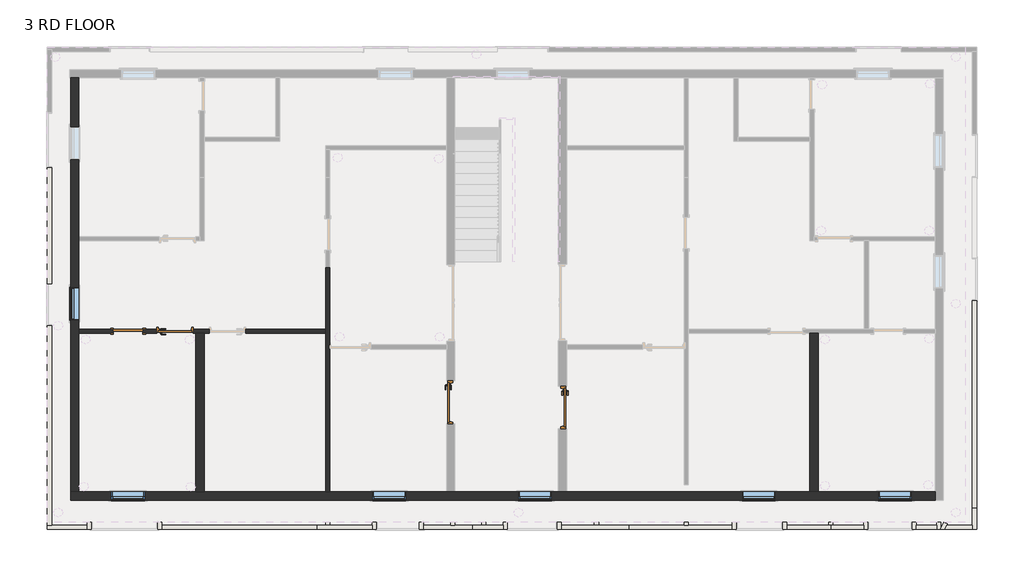
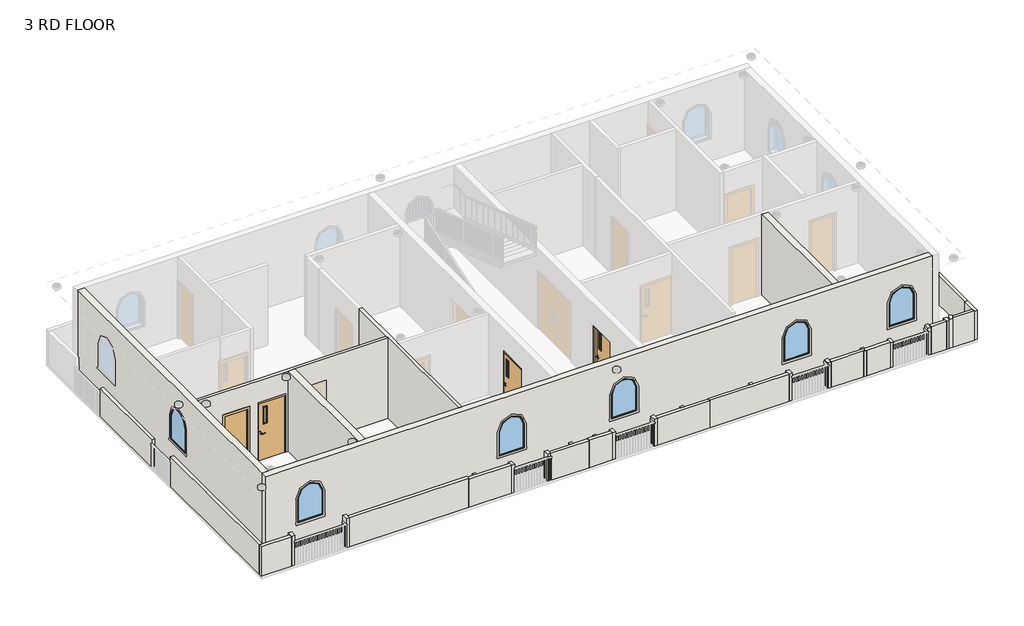
# One storey, part 1 of 7: 39 walls, 6 windows, 4 doors.
"""IFC4 building model written with IfcOpenShell, lengths in millimetres."""

from ifc_helpers import new_model, si_unit, frame, origin, place, context, project, spatial, polyline, circle_curve, outline, extrude, faceted_brep, transform, mapped, element, save
from ifc_brep_helpers import plane_surface, revolved_surface, advanced_brep
from components import door_586e558e, door_7d8f8091, door_passage_single_vision_lite_3_x7_38248cdf, door_d141acb4, window_fixed_round_top_3_x_4_dee2be1c

model = new_model("IFC4")

# Units and contexts
model_context = context("Model", 3, world=origin())
ifc_project = project(units=[si_unit("LENGTHUNIT", "METRE", prefix="MILLI")], contexts=[model_context])

# Site, building, storey
site = spatial("IfcSite", under=ifc_project)
building = spatial("IfcBuilding", under=site)
storey = spatial("IfcBuildingStorey", under=building, Name="3 RD FLOOR", Elevation=9601.2)

# Doors
placement = place(None, origin())
door_shape = door_586e558e(model_context)
element("IfcDoor", 1, ObjectType="Door-Passage-Single-Vision_Lite : 3'6\"X7' 2", at=placement, inside=storey, context=model_context, shape_type="MappedRepresentation", body=[
    mapped(door_shape, transform((1116.1432011, -1461.3932193, 9601.2), x_axis=(0.0, -1.0, 0.0), y_axis=(1.0, 0.0, 0.0), z_axis=(0.0, 0.0, 1.0))),
])
door_2_shape = door_7d8f8091(model_context)
element("IfcDoor", 2, ObjectType="Door-Passage-Single-Vision_Lite : 3'7\"X7' 3", at=placement, inside=storey, context=model_context, shape_type="MappedRepresentation", body=[
    mapped(door_2_shape, transform((-1956.7487998, -1318.7421379, 9601.2), x_axis=(0.0, -1.0, 0.0), y_axis=(1.0, 0.0, 0.0), z_axis=(0.0, 0.0, 1.0))),
])
door_passage_single_vision_lite_3_x7_shape = door_passage_single_vision_lite_3_x7_38248cdf(model_context)
element("IfcDoor", 3, ObjectType="Door-Passage-Single-Vision_Lite : 3'X7'", at=placement, inside=storey, context=model_context, shape_type="MappedRepresentation", body=[
    mapped(door_passage_single_vision_lite_3_x7_shape, transform((-9570.3987992, 646.8067334, 9601.2), x_axis=(1.0, 0.0, 0.0), y_axis=(0.0, 1.0, 0.0), z_axis=(0.0, 0.0, 1.0))),
])
door_3_shape = door_d141acb4(model_context)
element("IfcDoor", 4, ObjectType="Single-Flush : 2'8\"x 7'", at=placement, inside=storey, context=model_context, shape_type="MappedRepresentation", body=[
    mapped(door_3_shape, transform((-10865.7987992, 640.4567334, 9601.2), x_axis=(1.0, 0.0, 0.0), y_axis=(0.0, 1.0, 0.0), z_axis=(0.0, 0.0, 1.0))),
])

# Walls
element("IfcWall", 5, ObjectType="Generic - 4.5\"", at=placement, inside=storey, context=model_context, shape_type="Brep", body=[
    faceted_brep([(-10459.3987992, 583.3067334, 11734.8), (-10459.3987992, 583.3067334, 9601.2), (-10078.3987992, 583.3067334, 9601.2), (-10078.3987992, 583.3067334, 11836.4), (-9062.3987992, 583.3067334, 11836.4), (-9062.3987992, 583.3067334, 9601.2), (-8998.8987992, 583.3067334, 9601.2), (-8770.2987992, 583.3067334, 9601.2), (-8630.5987992, 583.3067334, 9601.2), (-8630.5987992, 583.3067334, 11836.4), (-7614.5987992, 583.3067334, 11836.4), (-7614.5987992, 583.3067334, 9601.2), (-5417.4987995, 583.3067334, 9601.2), (-5417.4987995, 583.3067334, 12649.2), (-8770.2987992, 583.3067334, 12649.2), (-8998.8987992, 583.3067334, 12649.2), (-12224.6987925, 583.3067334, 12649.2), (-12224.6987925, 583.3067334, 9601.2), (-11272.1987992, 583.3067334, 9601.2), (-11272.1987992, 583.3067334, 11734.8), (-10078.3987992, 697.6067334, 9601.2), (-10459.3987992, 697.6067334, 9601.2), (-10459.3987992, 697.6067334, 11734.8), (-11272.1987992, 697.6067334, 11734.8), (-11272.1987992, 697.6067334, 9601.2), (-12224.6987925, 697.6067334, 9601.2), (-12224.6987925, 697.6067334, 12649.2), (-5417.4987995, 697.6067334, 12649.2), (-5417.4987995, 697.6067334, 9601.2), (-7614.5987992, 697.6067334, 9601.2), (-7614.5987992, 697.6067334, 11836.4), (-8630.5987992, 697.6067334, 11836.4), (-8630.5987992, 697.6067334, 9601.2), (-9062.3987992, 697.6067334, 9601.2), (-9062.3987992, 697.6067334, 11836.4), (-10078.3987992, 697.6067334, 11836.4)], [[[0, 1, 2, 3, 4, 5, 6, 7, 8, 9, 10, 11, 12, 13, 14, 15, 16, 17, 18, 19]], [[20, 21, 22, 23, 24, 25, 26, 27, 28, 29, 30, 31, 32, 33, 34, 35]], [[28, 12, 11, 29]], [[32, 8, 7, 6, 5, 33]], [[18, 17, 25, 24]], [[2, 1, 21, 20]], [[16, 15, 14, 13, 27, 26]], [[17, 16, 26, 25]], [[13, 12, 28, 27]], [[9, 8, 32, 31]], [[10, 9, 31, 30]], [[11, 10, 30, 29]], [[4, 34, 33, 5]], [[34, 4, 3, 35]], [[35, 3, 2, 20]], [[22, 21, 1, 0]], [[23, 22, 0, 19]], [[24, 23, 19, 18]]]),
])
element("IfcWall", 6, ObjectType="Generic - 4.5\"", at=placement, inside=storey, context=model_context, shape_type="Brep", body=[
    faceted_brep([(-5417.4987995, 2399.4067802, 9601.2), (-5417.4987995, 697.6067334, 9601.2), (-5417.4987995, 583.3067334, 9601.2), (-5417.4987995, -3785.4932193, 9601.2), (-5417.4987995, -3785.4932193, 12649.2), (-5417.4987995, 583.3067334, 12649.2), (-5417.4987995, 697.6067334, 12649.2), (-5417.4987995, 2399.4067802, 12649.2), (-5303.1987995, 2399.4067802, 12649.2), (-5303.1987995, 262.4078621, 12649.2), (-5303.1987995, 148.1078621, 12649.2), (-5303.1987995, -3785.4932193, 12649.2), (-5303.1987995, -3785.4932193, 9601.2), (-5303.1987995, 148.1078621, 9601.2), (-5303.1987995, 148.1078621, 11836.4), (-5303.1987995, 262.4078621, 11836.4), (-5303.1987995, 262.4078621, 9601.2), (-5303.1987995, 2399.4067802, 9601.2), (-5334.9487995, 262.4078621, 9601.2), (-5334.9487995, 148.1078621, 9601.2), (-5334.9487995, 262.4078621, 11836.4), (-5334.9487995, 148.1078621, 11836.4)], [[[0, 1, 2, 3, 4, 5, 6, 7]], [[8, 9, 10, 11, 12, 13, 14, 15, 16, 17]], [[3, 2, 1, 0, 17, 16, 18, 19, 13, 12]], [[7, 6, 5, 4, 11, 10, 9, 8]], [[0, 7, 8, 17]], [[20, 18, 16, 15]], [[19, 21, 14, 13]], [[21, 20, 15, 14]], [[18, 20, 21, 19]], [[4, 3, 12, 11]]]),
])
element("IfcWall", 7, ObjectType="Generic - 4.5\"", at=placement, inside=storey, context=model_context, shape_type="Brep", body=[
    faceted_brep([(-13088.8067989, -4826.8932661, 9601.2), (-11996.6067989, -4826.8932661, 9601.2), (-11996.6067989, -4826.8932661, 10714.1417562), (-13088.8067989, -4826.8932661, 10714.1417562), (-13088.8067989, -4712.5932661, 9601.2), (-13088.8067989, -4712.5932661, 10714.1417562), (-11996.6067989, -4712.5932661, 10714.1417562), (-11996.6067989, -4712.5932661, 9601.2), (-12974.5067989, -4712.5932661, 9601.2)], [[[0, 1, 2, 3]], [[4, 5, 6, 7, 8]], [[1, 0, 4, 8, 7]], [[3, 2, 6, 5]], [[2, 1, 7, 6]], [[0, 3, 5, 4]]]),
])
element("IfcWall", 8, ObjectType="Generic - 4.5\"", at=placement, inside=storey, context=model_context, shape_type="Brep", body=[
    faceted_brep([(-11996.6067989, -4623.6932193, 9601.2), (-11996.6067989, -4712.5932661, 9601.2), (-11996.6067989, -4826.8932661, 9601.2), (-11996.6067989, -4826.8932661, 10714.1417562), (-11996.6067989, -4826.8932661, 10735.1303619), (-11996.6067989, -4623.6932193, 10735.1303619), (-11882.3067989, -4623.6932193, 9601.2), (-11882.3067989, -4623.6932193, 10735.1303619), (-11882.3067989, -4826.8932661, 10735.1303619), (-11882.3067989, -4826.8932661, 9601.2)], [[[0, 1, 2, 3, 4, 5]], [[6, 7, 8, 9]], [[2, 1, 0, 6, 9]], [[5, 4, 8, 7]], [[0, 5, 7, 6]], [[4, 3, 2, 9, 8]]]),
])
element("IfcWall", 9, ObjectType="Generic - 4.5\"", at=placement, inside=storey, context=model_context, shape_type="Brep", body=[
    faceted_brep([(11660.3143245, -4826.8932661, 9601.2), (12426.0012043, -4826.8932661, 9601.2), (12426.0012043, -4826.8932661, 10693.0617784), (12426.0012043, -4826.8932661, 10704.3196614), (11660.3143245, -4826.8932661, 10704.3196614), (11660.3143245, -4826.8932661, 10690.7342527), (11716.0621594, -4712.5932661, 9601.2), (11716.0621594, -4712.5932661, 10704.3196614), (12426.0012043, -4712.5932661, 10704.3196614), (12426.0012043, -4712.5932661, 9601.2)], [[[0, 1, 2, 3, 4, 5]], [[6, 7, 8, 9]], [[1, 0, 6, 9]], [[4, 3, 8, 7]], [[3, 2, 1, 9, 8]], [[0, 5, 4, 7, 6]]]),
])
element("IfcWall", 10, ObjectType="Generic - 4.5\"", at=placement, inside=storey, context=model_context, shape_type="Brep", body=[
    faceted_brep([(11632.2512075, -4623.6932193, 9601.2), (11533.1439227, -4826.8932661, 9601.2), (11533.1439227, -4826.8932661, 10690.7342527), (11632.2512075, -4623.6932193, 10690.7342527), (11734.983367, -4673.7990414, 9601.2), (11734.983367, -4673.7990414, 10690.7342527), (11660.3143245, -4826.8932661, 10690.7342527), (11660.3143245, -4826.8932661, 9601.2), (11716.0621594, -4712.5932661, 9601.2)], [[[0, 1, 2, 3]], [[4, 5, 6, 7, 8]], [[1, 0, 4, 8, 7]], [[3, 2, 6, 5]], [[0, 3, 5, 4]], [[2, 1, 7, 6]]]),
])
element("IfcWall", 11, ObjectType="Generic - 4.5\"", at=placement, inside=storey, context=model_context, shape_type="Brep", body=[
    faceted_brep([(12426.0012043, -4236.3432661, 9601.2), (12426.0012043, -4712.5932661, 9601.2), (12426.0012043, -4826.8932661, 9601.2), (12426.0012043, -4826.8932661, 10693.0617784), (12426.0012043, -4236.3432661, 10693.0617784), (12426.0012043, -4236.3432661, 10687.8712164), (12540.3012043, -4236.3432661, 9601.2), (12540.3012043, -4236.3432661, 10687.8712164), (12540.3012043, -4236.3432661, 10693.0617784), (12540.3012043, -4826.8932661, 10693.0617784), (12540.3012043, -4826.8932661, 9601.2)], [[[0, 1, 2, 3, 4, 5]], [[6, 7, 8, 9, 10]], [[2, 1, 0, 6, 10]], [[4, 3, 9, 8]], [[0, 5, 4, 8, 7, 6]], [[3, 2, 10, 9]]]),
])
element("IfcWall", 12, ObjectType="Generic - 4.5\"", at=placement, inside=storey, context=model_context, shape_type="SweptSolid", body=[
    extrude(outline(polyline([(-5417.4987995, -4712.5932661), (-5417.4987995, -4623.6932193), (-5303.1987995, -4623.6932193), (-5303.1987995, -4712.5932661), (-5417.4987995, -4712.5932661)])), frame((0.0, 0.0, 9601.2), z_axis=(0.0, 0.0, 1.0), x_axis=(1.0, 0.0, 0.0)), (0.0, 0.0, 1.0), 1063.0786215),
])
element("IfcWall", 13, ObjectType="Generic - 4.5\"", at=placement, inside=storey, context=model_context, shape_type="Brep", body=[
    faceted_brep([(-5663.8033402, -4826.8932661, 9601.2), (-4134.7987995, -4826.8932661, 9601.2), (-4134.7987995, -4826.8932661, 10660.3218247), (-4134.7987995, -4826.8932661, 10668.4575049), (-5663.8033402, -4826.8932661, 10668.4575049), (-5663.8033402, -4712.5932661, 9601.2), (-5663.8033402, -4712.5932661, 10668.4575049), (-4134.7987995, -4712.5932661, 10668.4575049), (-4134.7987995, -4712.5932661, 9601.2), (-5303.1987995, -4712.5932661, 9601.2), (-5417.4987995, -4712.5932661, 9601.2)], [[[0, 1, 2, 3, 4]], [[5, 6, 7, 8, 9, 10]], [[1, 0, 5, 10, 9, 8]], [[4, 3, 7, 6]], [[0, 4, 6, 5]], [[3, 2, 1, 8, 7]]]),
])
element("IfcWall", 14, ObjectType="Generic - 4.5\"", at=placement, inside=storey, context=model_context, shape_type="Brep", body=[
    faceted_brep([(-2725.0987995, -4826.8932661, 9601.2), (-1354.4417672, -4826.8932661, 9601.2), (-1354.4417672, -4826.8932661, 10617.2), (-2725.0987995, -4826.8932661, 10617.2), (-2725.0987995, -4712.5932661, 9601.2), (-2725.0987995, -4712.5932661, 10617.2), (-1354.4417672, -4712.5932661, 10617.2), (-1354.4417672, -4712.5932661, 9601.2), (-1848.7987998, -4712.5932661, 9601.2), (-1963.0987998, -4712.5932661, 9601.2)], [[[0, 1, 2, 3]], [[4, 5, 6, 7, 8, 9]], [[1, 0, 4, 9, 8, 7]], [[2, 1, 7, 6]], [[3, 2, 6, 5]], [[0, 3, 5, 4]]]),
])
element("IfcWall", 15, ObjectType="Generic - 4.5\"", at=placement, inside=storey, context=model_context, shape_type="SweptSolid", body=[
    extrude(outline(polyline([(-1963.0987998, -4712.5932661), (-1963.0987998, -4623.6932193), (-1848.7987998, -4623.6932193), (-1848.7987998, -4712.5932661), (-1963.0987998, -4712.5932661)])), frame((0.0, 0.0, 9601.2), z_axis=(0.0, 0.0, 1.0), x_axis=(1.0, 0.0, 0.0)), (0.0, 0.0, 1.0), 1029.3234006),
])
element("IfcWall", 16, ObjectType="Generic - 4.5\"", at=placement, inside=storey, context=model_context, shape_type="SweptSolid", body=[
    extrude(outline(polyline([(-1112.1987998, -4712.5932661), (-1112.1987998, -4623.6932193), (-997.8987998, -4623.6932193), (-997.8987998, -4712.5932661), (-1112.1987998, -4712.5932661)])), frame((0.0, 0.0, 9601.2), z_axis=(0.0, 0.0, 1.0), x_axis=(1.0, 0.0, 0.0)), (0.0, 0.0, 1.0), 1016.0),
])
element("IfcWall", 17, ObjectType="Generic - 4.5\"", at=placement, inside=storey, context=model_context, shape_type="SweptSolid", body=[
    extrude(outline(polyline([(1999.3012002, -4712.5932661), (1999.3012002, -4623.6932193), (2113.6012002, -4623.6932193), (2113.6012002, -4712.5932661), (1999.3012002, -4712.5932661)])), frame((0.0, 0.0, 9601.2), z_axis=(0.0, 0.0, 1.0), x_axis=(1.0, 0.0, 0.0)), (0.0, 0.0, 1.0), 1013.2250283),
])
element("IfcWall", 18, ObjectType="Generic - 4.5\"", at=placement, inside=storey, context=model_context, shape_type="SweptSolid", body=[
    extrude(outline(polyline([(4475.8012082, -4712.5932661), (4475.8012082, -4623.6932193), (4590.1012082, -4623.6932193), (4590.1012082, -4712.5932661), (4475.8012082, -4712.5932661)])), frame((0.0, 0.0, 9601.2), z_axis=(0.0, 0.0, 1.0), x_axis=(1.0, 0.0, 0.0)), (0.0, 0.0, 1.0), 1027.4591445),
])
element("IfcWall", 19, ObjectType="Generic - 4.5\"", at=placement, inside=storey, context=model_context, shape_type="Brep", body=[
    faceted_brep([(2962.6087812, -4826.8932661, 9601.2), (5802.9512082, -4826.8932661, 9601.2), (5802.9512082, -4826.8932661, 10628.6591445), (2962.6087812, -4826.8932661, 10628.6591445), (2962.6087812, -4826.8932661, 10614.4250283), (2962.6087812, -4712.5932661, 9601.2), (2962.6087812, -4712.5932661, 10614.4250283), (2962.6087812, -4712.5932661, 10628.6591445), (4475.8012082, -4712.5932661, 10628.6591445), (4590.1012082, -4712.5932661, 10628.6591445), (5802.9512082, -4712.5932661, 10628.6591445), (5802.9512082, -4712.5932661, 9601.2), (4590.1012082, -4712.5932661, 9601.2), (4475.8012082, -4712.5932661, 9601.2)], [[[0, 1, 2, 3, 4]], [[5, 6, 7, 8, 9, 10, 11, 12, 13]], [[1, 0, 5, 13, 12, 11]], [[3, 2, 10, 9, 8, 7]], [[0, 4, 3, 7, 6, 5]], [[2, 1, 11, 10]]]),
])
element("IfcWall", 20, ObjectType="Generic - 4.5\"", at=placement, inside=storey, context=model_context, shape_type="Brep", body=[
    faceted_brep([(5802.9512082, -4623.6932193, 9601.2), (5802.9512082, -4712.5932661, 9601.2), (5802.9512082, -4826.8932661, 9601.2), (5802.9512082, -4826.8932661, 10628.6591445), (5802.9512082, -4826.8932661, 10633.5822201), (5802.9512082, -4623.6932193, 10633.5822201), (5917.2512082, -4623.6932193, 9601.2), (5917.2512082, -4623.6932193, 10633.5822201), (5917.2512082, -4826.8932661, 10633.5822201), (5917.2512082, -4826.8932661, 9601.2)], [[[0, 1, 2, 3, 4, 5]], [[6, 7, 8, 9]], [[2, 1, 0, 6, 9]], [[5, 4, 8, 7]], [[0, 5, 7, 6]], [[4, 3, 2, 9, 8]]]),
])
element("IfcWall", 21, ObjectType="Generic - 4.5\"", at=placement, inside=storey, context=model_context, shape_type="Brep", body=[
    faceted_brep([(7190.3011643, -4623.6932193, 9601.2), (7190.3011643, -4826.8932661, 9601.2), (7190.3011643, -4826.8932661, 10574.0158009), (7190.3011643, -4623.6932193, 10574.0158009), (7304.6011643, -4623.6932193, 9601.2), (7304.6011643, -4623.6932193, 10574.0158009), (7304.6011643, -4712.5932661, 10574.0158009), (7304.6011643, -4826.8932661, 10574.0158009), (7304.6011643, -4826.8932661, 9601.2), (7304.6011643, -4712.5932661, 9601.2)], [[[0, 1, 2, 3]], [[4, 5, 6, 7, 8, 9]], [[1, 0, 4, 9, 8]], [[3, 2, 7, 6, 5]], [[0, 3, 5, 4]], [[2, 1, 8, 7]]]),
])
element("IfcWall", 22, ObjectType="Generic - 4.5\"", at=placement, inside=storey, context=model_context, shape_type="Brep", body=[
    faceted_brep([(7304.6011643, -4826.8932661, 9601.2), (8463.6012082, -4826.8932661, 9601.2), (8463.6012082, -4826.8932661, 10557.6159658), (8520.7512082, -4826.8932661, 10557.6159658), (8520.7512082, -4826.8932661, 10570.880309), (8520.7512082, -4826.8932661, 10574.1581334), (7304.6011643, -4826.8932661, 10574.1581334), (7304.6011643, -4712.5932661, 9601.2), (7304.6011643, -4712.5932661, 10574.1581334), (8520.7512082, -4712.5932661, 10574.1581334), (8520.7512082, -4712.5932661, 10570.880309), (8520.7512082, -4712.5932661, 10557.6159658), (8463.6012082, -4712.5932661, 10557.6159658), (8463.6012082, -4712.5932661, 9601.2)], [[[0, 1, 2, 3, 4, 5, 6]], [[7, 8, 9, 10, 11, 12, 13]], [[1, 0, 7, 13]], [[6, 5, 9, 8]], [[0, 6, 8, 7]], [[5, 4, 3, 11, 10, 9]], [[11, 3, 2, 12]], [[2, 1, 13, 12]]]),
])
element("IfcWall", 23, ObjectType="Generic - 4.5\"", at=placement, inside=storey, context=model_context, shape_type="Brep", body=[
    faceted_brep([(8463.6012082, -4623.6932193, 9601.2), (8463.6012082, -4712.5932661, 9601.2), (8463.6012082, -4826.8932661, 9601.2), (8463.6012082, -4826.8932661, 10557.6159658), (8463.6012082, -4712.5932661, 10557.6159658), (8463.6012082, -4623.6932193, 10557.6159658), (8577.9012082, -4623.6932193, 9601.2), (8577.9012082, -4623.6932193, 10557.6159658), (8577.9012082, -4712.5932661, 10557.6159658), (8577.9012082, -4826.8932661, 10557.6159658), (8577.9012082, -4826.8932661, 9601.2), (8577.9012082, -4712.5932661, 9601.2), (8520.7512082, -4826.8932661, 10557.6159658)], [[[0, 1, 2, 3, 4, 5]], [[6, 7, 8, 9, 10, 11]], [[2, 1, 0, 6, 11, 10]], [[5, 4, 3, 12, 9, 8, 7]], [[0, 5, 7, 6]], [[3, 2, 10, 9, 12]]]),
])
element("IfcWall", 24, ObjectType="Generic - 4.5\"", at=placement, inside=storey, context=model_context, shape_type="Brep", body=[
    faceted_brep([(8577.9012082, -4826.8932661, 9601.2), (9422.4512082, -4826.8932661, 9601.2), (9422.4512082, -4826.8932661, 10553.4060641), (9422.4512082, -4826.8932661, 10570.880309), (8520.7512082, -4826.8932661, 10570.880309), (8520.7512082, -4826.8932661, 10557.6159658), (8577.9012082, -4826.8932661, 10557.6159658), (8577.9012082, -4712.5932661, 9601.2), (8577.9012082, -4712.5932661, 10557.6159658), (8520.7512082, -4712.5932661, 10557.6159658), (8520.7512082, -4712.5932661, 10570.880309), (9422.4512082, -4712.5932661, 10570.880309), (9422.4512082, -4712.5932661, 9601.2)], [[[0, 1, 2, 3, 4, 5, 6]], [[7, 8, 9, 10, 11, 12]], [[1, 0, 7, 12]], [[4, 3, 11, 10]], [[3, 2, 1, 12, 11]], [[5, 4, 10, 9]], [[5, 9, 8, 6]], [[0, 6, 8, 7]]]),
])
element("IfcWall", 25, ObjectType="Generic - 4.5\"", at=placement, inside=storey, context=model_context, shape_type="Brep", body=[
    faceted_brep([(9422.4512082, -4623.6932193, 9601.2), (9422.4512082, -4712.5932661, 9601.2), (9422.4512082, -4826.8932661, 9601.2), (9422.4512082, -4826.8932661, 10553.4060641), (9422.4512082, -4623.6932193, 10553.4060641), (9536.7512082, -4623.6932193, 9601.2), (9536.7512082, -4623.6932193, 10553.4060641), (9536.7512082, -4826.8932661, 10553.4060641), (9536.7512082, -4826.8932661, 9601.2)], [[[0, 1, 2, 3, 4]], [[5, 6, 7, 8]], [[2, 1, 0, 5, 8]], [[4, 3, 7, 6]], [[0, 4, 6, 5]], [[3, 2, 8, 7]]]),
])
element("IfcWall", 26, ObjectType="Generic - 4.5\"", at=placement, inside=storey, context=model_context, shape_type="Brep", body=[
    faceted_brep([(10764.1617205, -4623.6932193, 9601.2), (10764.1617205, -4826.8932661, 9601.2), (10764.1617205, -4826.8932661, 10627.5072304), (10764.1617205, -4623.6932193, 10627.5072304), (10878.4617205, -4623.6932193, 9601.2), (10878.4617205, -4623.6932193, 10627.5072304), (10878.4617205, -4826.8932661, 10627.5072304), (10878.4617205, -4826.8932661, 9601.2), (10878.4617205, -4712.5932661, 9601.2)], [[[0, 1, 2, 3]], [[4, 5, 6, 7, 8]], [[1, 0, 4, 8, 7]], [[3, 2, 6, 5]], [[0, 3, 5, 4]], [[2, 1, 7, 6]]]),
])
element("IfcWall", 27, ObjectType="Generic - 4.5\"", at=placement, inside=storey, context=model_context, shape_type="Brep", body=[
    faceted_brep([(10878.4617205, -4826.8932661, 9601.2), (11437.2617205, -4826.8932661, 9601.2), (11437.2617205, -4826.8932661, 10649.8912221), (10878.4617205, -4826.8932661, 10649.8912221), (10878.4617205, -4826.8932661, 10627.5072304), (10878.4617205, -4712.5932661, 9601.2), (10878.4617205, -4712.5932661, 10649.8912221), (11437.2617205, -4712.5932661, 10649.8912221), (11437.2617205, -4712.5932661, 9601.2)], [[[0, 1, 2, 3, 4]], [[5, 6, 7, 8]], [[1, 0, 5, 8]], [[3, 2, 7, 6]], [[0, 4, 3, 6, 5]], [[2, 1, 8, 7]]]),
])
element("IfcWall", 28, ObjectType="Generic - 4.5\"", at=placement, inside=storey, context=model_context, shape_type="Brep", body=[
    faceted_brep([(11437.2617205, -4623.6932193, 9601.2), (11437.2617205, -4712.5932661, 9601.2), (11437.2617205, -4826.8932661, 9601.2), (11437.2617205, -4826.8932661, 10649.8912221), (11437.2617205, -4712.5932661, 10649.8912221), (11437.2617205, -4623.6932193, 10649.8912221), (11551.5617205, -4623.6932193, 9601.2), (11551.5617205, -4623.6932193, 10649.8912221), (11551.5617205, -4826.8932661, 10649.8912221), (11551.5617205, -4826.8932661, 9601.2)], [[[0, 1, 2, 3, 4, 5]], [[6, 7, 8, 9]], [[2, 1, 0, 6, 9]], [[5, 4, 3, 8, 7]], [[0, 5, 7, 6]], [[3, 2, 9, 8]]]),
])
element("IfcWall", 29, ObjectType="Generic - 4.5\"", at=placement, inside=storey, context=model_context, shape_type="Brep", body=[
    faceted_brep([(-4134.7987995, -4623.6932193, 9601.2), (-4134.7987995, -4712.5932661, 9601.2), (-4134.7987995, -4826.8932661, 9601.2), (-4134.7987995, -4826.8932661, 10660.3218247), (-4134.7987995, -4623.6932193, 10660.3218247), (-4020.4987995, -4623.6932193, 9601.2), (-4020.4987995, -4623.6932193, 10660.3218247), (-4020.4987995, -4826.8932661, 10660.3218247), (-4020.4987995, -4826.8932661, 9601.2)], [[[0, 1, 2, 3, 4]], [[5, 6, 7, 8]], [[2, 1, 0, 5, 8]], [[4, 3, 7, 6]], [[0, 4, 6, 5]], [[3, 2, 8, 7]]]),
])
element("IfcWall", 30, ObjectType="Generic - 4.5\"", at=placement, inside=storey, context=model_context, shape_type="Brep", body=[
    faceted_brep([(-2839.3987995, -4623.6932193, 9601.2), (-2839.3987995, -4826.8932661, 9601.2), (-2839.3987995, -4826.8932661, 10617.9549618), (-2839.3987995, -4623.6932193, 10617.9549618), (-2725.0987995, -4623.6932193, 9601.2), (-2725.0987995, -4623.6932193, 10617.9549618), (-2725.0987995, -4826.8932661, 10617.9549618), (-2725.0987995, -4826.8932661, 10617.2), (-2725.0987995, -4826.8932661, 9601.2), (-2725.0987995, -4712.5932661, 9601.2)], [[[0, 1, 2, 3]], [[4, 5, 6, 7, 8, 9]], [[1, 0, 4, 9, 8]], [[3, 2, 6, 5]], [[0, 3, 5, 4]], [[2, 1, 8, 7, 6]]]),
])
element("IfcWall", 31, ObjectType="Generic - 4.5\"", at=placement, inside=storey, context=model_context, shape_type="Brep", body=[
    faceted_brep([(-1354.4417672, -4826.8932661, 9601.2), (-520.5065315, -4826.8932661, 9601.2), (-520.5065315, -4826.8932661, 10625.0796817), (-520.5065315, -4826.8932661, 10632.340074), (-1354.4417672, -4826.8932661, 10632.340074), (-1354.4417672, -4826.8932661, 10617.2), (-1354.4417672, -4712.5932661, 9601.2), (-1354.4417672, -4712.5932661, 10617.2), (-1354.4417672, -4712.5932661, 10632.340074), (-520.5065315, -4712.5932661, 10632.340074), (-520.5065315, -4712.5932661, 9601.2), (-997.8987998, -4712.5932661, 9601.2), (-1112.1987998, -4712.5932661, 9601.2)], [[[0, 1, 2, 3, 4, 5]], [[6, 7, 8, 9, 10, 11, 12]], [[1, 0, 6, 12, 11, 10]], [[4, 3, 9, 8]], [[0, 5, 4, 8, 7, 6]], [[3, 2, 1, 10, 9]]]),
])
element("IfcWall", 32, ObjectType="Generic - 4.5\"", at=placement, inside=storey, context=model_context, shape_type="Brep", body=[
    faceted_brep([(-520.5065315, -4623.6932193, 9601.2), (-520.5065315, -4712.5932661, 9601.2), (-520.5065315, -4826.8932661, 9601.2), (-520.5065315, -4826.8932661, 10625.0796817), (-520.5065315, -4623.6932193, 10625.0796817), (-406.2065315, -4623.6932193, 9601.2), (-406.2065315, -4623.6932193, 10625.0796817), (-406.2065315, -4826.8932661, 10625.0796817), (-406.2065315, -4826.8932661, 9601.2)], [[[0, 1, 2, 3, 4]], [[5, 6, 7, 8]], [[2, 1, 0, 5, 8]], [[4, 3, 7, 6]], [[0, 4, 6, 5]], [[3, 2, 8, 7]]]),
])
element("IfcWall", 33, ObjectType="Generic - 4.5\"", at=placement, inside=storey, context=model_context, shape_type="Brep", body=[
    faceted_brep([(970.0932011, -4623.6932193, 9601.2), (970.0932011, -4826.8932661, 9601.2), (970.0932011, -4826.8932661, 10614.4250283), (970.0932011, -4623.6932193, 10614.4250283), (1084.3932011, -4623.6932193, 9601.2), (1084.3932011, -4623.6932193, 10614.4250283), (1084.3932011, -4712.5932661, 10614.4250283), (1084.3932011, -4826.8932661, 10614.4250283), (1084.3932011, -4826.8932661, 9601.2), (1084.3932011, -4712.5932661, 9601.2)], [[[0, 1, 2, 3]], [[4, 5, 6, 7, 8, 9]], [[1, 0, 4, 9, 8]], [[3, 2, 7, 6, 5]], [[0, 3, 5, 4]], [[2, 1, 8, 7]]]),
])
element("IfcWall", 34, ObjectType="Generic - 4.5\"", at=placement, inside=storey, context=model_context, shape_type="Brep", body=[
    faceted_brep([(1084.3932011, -4826.8932661, 9601.2), (2962.6087812, -4826.8932661, 9601.2), (2962.6087812, -4826.8932661, 10614.4250283), (1084.3932011, -4826.8932661, 10614.4250283), (1084.3932011, -4712.5932661, 9601.2), (1084.3932011, -4712.5932661, 10614.4250283), (1999.3012002, -4712.5932661, 10614.4250283), (2113.6012002, -4712.5932661, 10614.4250283), (2962.6087812, -4712.5932661, 10614.4250283), (2962.6087812, -4712.5932661, 9601.2), (2113.6012002, -4712.5932661, 9601.2), (1999.3012002, -4712.5932661, 9601.2)], [[[0, 1, 2, 3]], [[4, 5, 6, 7, 8, 9, 10, 11]], [[1, 0, 4, 11, 10, 9]], [[2, 1, 9, 8]], [[3, 2, 8, 7, 6, 5]], [[0, 3, 5, 4]]]),
])
element("IfcWall", 35, ObjectType="Generic - 4.5\"", at=placement, inside=storey, context=model_context, shape_type="Brep", body=[
    faceted_brep([(-10045.9470335, -4623.6932193, 9601.2), (-10045.9470335, -4826.8932661, 9601.2), (-10045.9470335, -4826.8932661, 10708.904535), (-10045.9470335, -4623.6932193, 10708.904535), (-9931.6470335, -4623.6932193, 9601.2), (-9931.6470335, -4623.6932193, 10708.904535), (-9931.6470335, -4712.5932661, 10708.904535), (-9931.6470335, -4826.8932661, 10708.904535), (-9931.6470335, -4826.8932661, 9601.2), (-9931.6470335, -4712.5932661, 9601.2)], [[[0, 1, 2, 3]], [[4, 5, 6, 7, 8, 9]], [[1, 0, 4, 9, 8]], [[3, 2, 7, 6, 5]], [[0, 3, 5, 4]], [[2, 1, 8, 7]]]),
])
element("IfcWall", 36, ObjectType="Generic - 4.5\"", at=placement, inside=storey, context=model_context, shape_type="Brep", body=[
    faceted_brep([(-9931.6470335, -4826.8932661, 9601.2), (-5663.8033402, -4826.8932661, 9601.2), (-5663.8033402, -4826.8932661, 10668.4575049), (-5663.8033402, -4826.8932661, 10708.904535), (-9931.6470335, -4826.8932661, 10708.904535), (-9931.6470335, -4712.5932661, 9601.2), (-9931.6470335, -4712.5932661, 10708.904535), (-5663.8033402, -4712.5932661, 10708.904535), (-5663.8033402, -4712.5932661, 10668.4575049), (-5663.8033402, -4712.5932661, 9601.2)], [[[0, 1, 2, 3, 4]], [[5, 6, 7, 8, 9]], [[1, 0, 5, 9]], [[3, 2, 1, 9, 8, 7]], [[4, 3, 7, 6]], [[0, 4, 6, 5]]]),
])
element("IfcWall", 37, ObjectType="Generic - 4.5\"", at=placement, inside=storey, context=model_context, shape_type="Brep", body=[
    faceted_brep([(-13088.8067989, 792.8567339, 9601.2), (-13088.8067989, -4712.5932661, 9601.2), (-13088.8067989, -4712.5932661, 10714.1417562), (-13088.8067989, -4712.5932661, 10715.367936), (-13088.8067989, 792.8567339, 10715.367936), (-12974.5067989, 792.8567339, 9601.2), (-12974.5067989, 792.8567339, 10715.367936), (-12974.5067989, -4712.5932661, 10715.367936), (-12974.5067989, -4712.5932661, 9601.2)], [[[0, 1, 2, 3, 4]], [[5, 6, 7, 8]], [[1, 0, 5, 8]], [[4, 3, 7, 6]], [[0, 4, 6, 5]], [[3, 2, 1, 8, 7]]]),
])
element("IfcWall", 38, ObjectType="Generic - 4.5\"", at=placement, inside=storey, context=model_context, shape_type="SweptSolid", body=[
    extrude(outline(polyline([(-12976.0338648, 5154.3604213), (-12976.0338648, 1953.9604213), (-13090.3338648, 1953.9604213), (-13090.3338648, 5154.3604213), (-12976.0338648, 5154.3604213)])), frame((0.0, 0.0, 9601.2), z_axis=(0.0, 0.0, 1.0), x_axis=(1.0, 0.0, 0.0)), (0.0, 0.0, 1.0), 1047.4413329),
])
element("IfcWall", 39, ObjectType="Generic - 4.5\"", at=placement, inside=storey, context=model_context, shape_type="SweptSolid", body=[
    extrude(outline(polyline([(12426.0012043, -4236.3432661), (12426.0012043, 1478.6567334), (12540.3012043, 1478.6567334), (12540.3012043, -4236.3432661), (12426.0012043, -4236.3432661)])), frame((0.0, 0.0, 9601.2), z_axis=(0.0, 0.0, 1.0), x_axis=(1.0, 0.0, 0.0)), (0.0, 0.0, 1.0), 1086.6712164),
])
element("IfcWall", 40, ObjectType="Generic - 9\"", at=placement, inside=storey, context=model_context, shape_type="AdvancedBrep", body=[
    advanced_brep(
    [(11397.3012075, -3785.4932193, 9601.2), (8171.5012079, -3785.4932193, 9601.2), (7942.9012079, -3785.4932193, 9601.2), (1236.7932011, -3785.4932193, 9601.2), (1008.1932011, -3785.4932193, 9601.2), (-1848.7987998, -3785.4932193, 9601.2), (-2077.3987998, -3785.4932193, 9601.2), (-5303.1987995, -3785.4932193, 9601.2), (-5417.4987995, -3785.4932193, 9601.2), (-8770.2987992, -3785.4932193, 9601.2), (-8998.8987992, -3785.4932193, 9601.2), (-12224.6987925, -3785.4932193, 9601.2), (-12453.2987925, -3785.4932193, 9601.2), (-12453.2987925, -3785.4932193, 12649.2), (-12224.6987925, -3785.4932193, 12649.2), (-8998.8987992, -3785.4932193, 12649.2), (-8770.2987992, -3785.4932193, 12649.2), (-5417.4987995, -3785.4932193, 12649.2), (-5303.1987995, -3785.4932193, 12649.2), (-2077.3987998, -3785.4932193, 12649.2), (-1848.7987998, -3785.4932193, 12649.2), (1008.1932011, -3785.4932193, 12649.2), (1236.7932011, -3785.4932193, 12649.2), (7942.9012079, -3785.4932193, 12649.2), (8171.5012079, -3785.4932193, 12649.2), (11397.3012075, -3785.4932193, 12649.2), (-10408.5987925, -3785.4932193, 10515.6), (-10408.5987925, -3785.4932193, 11430.0), (-11322.9987925, -3785.4932193, 11430.0), (-11322.9987925, -3785.4932193, 10515.6), (-3204.5237997, -3785.4932193, 10515.6), (-3204.5237997, -3785.4932193, 11430.0), (-4118.9237997, -3785.4932193, 11430.0), (-4118.9237997, -3785.4932193, 10515.6), (817.6932011, -3785.4932193, 10515.6), (817.6932011, -3785.4932193, 11430.0), (-96.7067989, -3785.4932193, 11430.0), (-96.7067989, -3785.4932193, 10515.6), (6990.4012079, -3785.4932193, 10515.6), (6990.4012079, -3785.4932193, 11430.0), (6076.0012079, -3785.4932193, 11430.0), (6076.0012079, -3785.4932193, 10515.6), (10749.6012075, -3785.4932193, 10515.6), (10749.6012075, -3785.4932193, 11430.0), (9835.2012075, -3785.4932193, 11430.0), (9835.2012075, -3785.4932193, 10515.6), (11397.3012075, -4014.0932193, 9601.2), (11397.3012075, -4014.0932193, 12649.2), (-12453.2987925, -4014.0932193, 12649.2), (-12453.2987925, -4014.0932193, 9601.2), (-10408.5987925, -4014.0932193, 10515.6), (-11322.9987925, -4014.0932193, 10515.6), (-11322.9987925, -4014.0932193, 11430.0), (-10408.5987925, -4014.0932193, 11430.0), (-3204.5237997, -4014.0932193, 10515.6), (-4118.9237997, -4014.0932193, 10515.6), (-4118.9237997, -4014.0932193, 11430.0), (-3204.5237997, -4014.0932193, 11430.0), (817.6932011, -4014.0932193, 10515.6), (-96.7067989, -4014.0932193, 10515.6), (-96.7067989, -4014.0932193, 11430.0), (817.6932011, -4014.0932193, 11430.0), (6990.4012079, -4014.0932193, 10515.6), (6076.0012079, -4014.0932193, 10515.6), (6076.0012079, -4014.0932193, 11430.0), (6990.4012079, -4014.0932193, 11430.0), (10749.6012075, -4014.0932193, 10515.6), (9835.2012075, -4014.0932193, 10515.6), (9835.2012075, -4014.0932193, 11430.0), (10749.6012075, -4014.0932193, 11430.0)],
    [
        (0, 1),
        (1, 2),
        (2, 3),
        (3, 4),
        (4, 5),
        (5, 6),
        (6, 7),
        (7, 8),
        (8, 9),
        (9, 10),
        (10, 11),
        (11, 12),
        (12, 13),
        (13, 14),
        (14, 15),
        (15, 16),
        (16, 17),
        (17, 18),
        (18, 19),
        (19, 20),
        (20, 21),
        (21, 22),
        (22, 23),
        (23, 24),
        (24, 25),
        (25, 0),
        (26, 27),
        (27, 28, circle_curve(frame((-10865.7987925, -3785.4932193, 11430.0), z_axis=(0.0, -1.0, 0.0), x_axis=(-1.0, 0.0, 0.0)), 457.2)),
        (28, 29),
        (29, 26),
        (30, 31),
        (31, 32, circle_curve(frame((-3661.7237997, -3785.4932193, 11430.0), z_axis=(0.0, -1.0, 0.0), x_axis=(-1.0, 0.0, 0.0)), 457.2)),
        (32, 33),
        (33, 30),
        (34, 35),
        (35, 36, circle_curve(frame((360.4932011, -3785.4932193, 11430.0), z_axis=(0.0, -1.0, 0.0), x_axis=(-1.0, 0.0, 0.0)), 457.2)),
        (36, 37),
        (37, 34),
        (38, 39),
        (39, 40, circle_curve(frame((6533.2012079, -3785.4932193, 11430.0), z_axis=(0.0, -1.0, 0.0), x_axis=(-1.0, 0.0, 0.0)), 457.2)),
        (40, 41),
        (41, 38),
        (42, 43),
        (43, 44, circle_curve(frame((10292.4012075, -3785.4932193, 11430.0), z_axis=(0.0, -1.0, 0.0), x_axis=(-1.0, 0.0, 0.0)), 457.2)),
        (44, 45),
        (45, 42),
        (46, 47),
        (47, 48),
        (48, 49),
        (49, 46),
        (50, 51),
        (51, 52),
        (52, 53, circle_curve(frame((-10865.7987925, -4014.0932193, 11430.0), z_axis=(0.0, 1.0, 0.0), x_axis=(-1.0, 0.0, 0.0)), 457.2)),
        (53, 50),
        (54, 55),
        (55, 56),
        (56, 57, circle_curve(frame((-3661.7237997, -4014.0932193, 11430.0), z_axis=(0.0, 1.0, 0.0), x_axis=(-1.0, 0.0, 0.0)), 457.2)),
        (57, 54),
        (58, 59),
        (59, 60),
        (60, 61, circle_curve(frame((360.4932011, -4014.0932193, 11430.0), z_axis=(0.0, 1.0, 0.0), x_axis=(-1.0, 0.0, 0.0)), 457.2)),
        (61, 58),
        (62, 63),
        (63, 64),
        (64, 65, circle_curve(frame((6533.2012079, -4014.0932193, 11430.0), z_axis=(0.0, 1.0, 0.0), x_axis=(-1.0, 0.0, 0.0)), 457.2)),
        (65, 62),
        (66, 67),
        (67, 68),
        (68, 69, circle_curve(frame((10292.4012075, -4014.0932193, 11430.0), z_axis=(0.0, 1.0, 0.0), x_axis=(-1.0, 0.0, 0.0)), 457.2)),
        (69, 66),
        (0, 46),
        (49, 12),
        (13, 48),
        (47, 25),
        (50, 26),
        (29, 51),
        (28, 52),
        (27, 53),
        (54, 30),
        (33, 55),
        (32, 56),
        (31, 57),
        (58, 34),
        (37, 59),
        (36, 60),
        (35, 61),
        (62, 38),
        (41, 63),
        (40, 64),
        (39, 65),
        (66, 42),
        (45, 67),
        (44, 68),
        (43, 69),
    ],
    [
        plane_surface(frame((11386.6090247, -3785.4932193, 9601.2), z_axis=(0.0, 1.0, 0.0), x_axis=(-1.0, 0.0, 0.0))),
        plane_surface(frame((11386.6090247, -4014.0932193, 9601.2), z_axis=(0.0, -1.0, 0.0), x_axis=(1.0, 0.0, 0.0))),
        plane_surface(frame((11511.6012075, -3785.4932193, 9601.2), z_axis=(0.0, 0.0, -1.0), x_axis=(0.0, -1.0, 0.0))),
        plane_surface(frame((-12338.9987925, -3785.4932193, 12649.2), z_axis=(0.0, 0.0, 1.0), x_axis=(0.0, -1.0, 0.0))),
        plane_surface(frame((11397.3012075, 7629.6366753, 9601.2), z_axis=(1.0, 0.0, 0.0), x_axis=(0.0, -1.0, 0.0))),
        plane_surface(frame((-12453.2987925, -3782.6829884, 9601.2), z_axis=(-1.0, 0.0, 0.0), x_axis=(0.0, -1.0, 0.0))),
        plane_surface(frame((-10408.5987925, -4014.0932193, 10515.6), z_axis=(0.0, 0.0, 1.0), x_axis=(0.0, 1.0, 0.0))),
        plane_surface(frame((-11322.9987925, -4014.0932193, 10515.6), z_axis=(1.0, 0.0, 0.0), x_axis=(0.0, 1.0, 0.0))),
        revolved_surface(polyline([(-11322.9987925, -3785.4932193, 11430.0), (-11322.9987925, -4014.0932193, 11430.0)]), (-10865.7987925, -3785.4932193, 11430.0), (0.0, 1.0, 0.0)),
        plane_surface(frame((-10408.5987925, -4014.0932193, 11430.0), z_axis=(-1.0, 0.0, 0.0), x_axis=(0.0, 1.0, 0.0))),
        plane_surface(frame((-3204.5237997, -4014.0932193, 10515.6), z_axis=(0.0, 0.0, 1.0), x_axis=(0.0, 1.0, 0.0))),
        plane_surface(frame((-4118.9237997, -4014.0932193, 10515.6), z_axis=(1.0, 0.0, 0.0), x_axis=(0.0, 1.0, 0.0))),
        revolved_surface(polyline([(-4118.9237997, -3785.4932193, 11430.0), (-4118.9237997, -4014.0932193, 11430.0)]), (-3661.7237997, -3785.4932193, 11430.0), (0.0, 1.0, 0.0)),
        plane_surface(frame((-3204.5237997, -4014.0932193, 11430.0), z_axis=(-1.0, 0.0, 0.0), x_axis=(0.0, 1.0, 0.0))),
        plane_surface(frame((817.6932011, -4014.0932193, 10515.6), z_axis=(0.0, 0.0, 1.0), x_axis=(0.0, 1.0, 0.0))),
        plane_surface(frame((-96.7067989, -4014.0932193, 10515.6), z_axis=(1.0, 0.0, 0.0), x_axis=(0.0, 1.0, 0.0))),
        revolved_surface(polyline([(-96.70679889999997, -3785.4932193, 11430.0), (-96.70679889999997, -4014.0932193, 11430.0)]), (360.4932011, -3785.4932193, 11430.0), (0.0, 1.0, 0.0)),
        plane_surface(frame((817.6932011, -4014.0932193, 11430.0), z_axis=(-1.0, 0.0, 0.0), x_axis=(0.0, 1.0, 0.0))),
        plane_surface(frame((6990.4012079, -4014.0932193, 10515.6), z_axis=(0.0, 0.0, 1.0), x_axis=(0.0, 1.0, 0.0))),
        plane_surface(frame((6076.0012079, -4014.0932193, 10515.6), z_axis=(1.0, 0.0, 0.0), x_axis=(0.0, 1.0, 0.0))),
        revolved_surface(polyline([(6076.0012079, -3785.4932193, 11430.0), (6076.0012079, -4014.0932193, 11430.0)]), (6533.2012079, -3785.4932193, 11430.0), (0.0, 1.0, 0.0)),
        plane_surface(frame((6990.4012079, -4014.0932193, 11430.0), z_axis=(-1.0, 0.0, 0.0), x_axis=(0.0, 1.0, 0.0))),
        plane_surface(frame((10749.6012075, -4014.0932193, 10515.6), z_axis=(0.0, 0.0, 1.0), x_axis=(0.0, 1.0, 0.0))),
        plane_surface(frame((9835.2012075, -4014.0932193, 10515.6), z_axis=(1.0, 0.0, 0.0), x_axis=(0.0, 1.0, 0.0))),
        revolved_surface(polyline([(9835.201207499998, -3785.4932193, 11430.0), (9835.201207499998, -4014.0932193, 11430.0)]), (10292.4012075, -3785.4932193, 11430.0), (0.0, 1.0, 0.0)),
        plane_surface(frame((10749.6012075, -4014.0932193, 11430.0), z_axis=(-1.0, 0.0, 0.0), x_axis=(0.0, 1.0, 0.0))),
    ],
    [
        (0, [[1, 2, 3, 4, 5, 6, 7, 8, 9, 10, 11, 12, 13, 14, 15, 16, 17, 18, 19, 20, 21, 22, 23, 24, 25, 26], [27, 28, 29, 30], [31, 32, 33, 34], [35, 36, 37, 38], [39, 40, 41, 42], [43, 44, 45, 46]]),
        (1, [[47, 48, 49, 50], [51, 52, 53, 54], [55, 56, 57, 58], [59, 60, 61, 62], [63, 64, 65, 66], [67, 68, 69, 70]]),
        (2, [[-12, -11, -10, -9, -8, -7, -6, -5, -4, -3, -2, -1, 71, -50, 72]]),
        (3, [[-25, -24, -23, -22, -21, -20, -19, -18, -17, -16, -15, -14, 73, -48, 74]]),
        (4, [[-26, -74, -47, -71]]),
        (5, [[-13, -72, -49, -73]]),
        (6, [[-51, 75, -30, 76]]),
        (7, [[-52, -76, -29, 77]]),
        (8, [[-53, -77, -28, 78]]),
        (9, [[-54, -78, -27, -75]]),
        (10, [[-55, 79, -34, 80]]),
        (11, [[-56, -80, -33, 81]]),
        (12, [[-57, -81, -32, 82]]),
        (13, [[-58, -82, -31, -79]]),
        (14, [[-59, 83, -38, 84]]),
        (15, [[-60, -84, -37, 85]]),
        (16, [[-61, -85, -36, 86]]),
        (17, [[-62, -86, -35, -83]]),
        (18, [[-63, 87, -42, 88]]),
        (19, [[-64, -88, -41, 89]]),
        (20, [[-65, -89, -40, 90]]),
        (21, [[-66, -90, -39, -87]]),
        (22, [[-67, 91, -46, 92]]),
        (23, [[-68, -92, -45, 93]]),
        (24, [[-69, -93, -44, 94]]),
        (25, [[-70, -94, -43, -91]]),
    ],
),
])
element("IfcWall", 41, ObjectType="Generic - 9\"", at=placement, inside=storey, context=model_context, shape_type="AdvancedBrep", body=[
    advanced_brep(
    [(-12224.6987925, -3785.4932193, 9601.2), (-12224.6987925, 583.3067334, 9601.2), (-12224.6987925, 697.6067334, 9601.2), (-12224.6987925, 3136.0067332, 9601.2), (-12224.6987925, 3250.3067332, 9601.2), (-12224.6987925, 7631.8067329, 9601.2), (-12224.6987925, 7631.8067329, 12649.2), (-12224.6987925, 3250.3067332, 12649.2), (-12224.6987925, 3136.0067332, 12649.2), (-12224.6987925, 697.6067334, 12649.2), (-12224.6987925, 583.3067334, 12649.2), (-12224.6987925, -3785.4932193, 12649.2), (-12224.6987925, 5368.031733, 10515.6), (-12224.6987925, 5368.031733, 11430.0), (-12224.6987925, 6282.431733, 11430.0), (-12224.6987925, 6282.431733, 10515.6), (-12224.6987925, 945.2567334, 10515.6), (-12224.6987925, 945.2567334, 11430.0), (-12224.6987925, 1859.6567334, 11430.0), (-12224.6987925, 1859.6567334, 10515.6), (-12453.2987925, -3785.4932193, 9601.2), (-12453.2987925, -3785.4932193, 12649.2), (-12453.2987925, 7631.8067329, 12649.2), (-12453.2987925, 7631.8067329, 9601.2), (-12453.2987925, 5368.031733, 10515.6), (-12453.2987925, 6282.431733, 10515.6), (-12453.2987925, 6282.431733, 11430.0), (-12453.2987925, 5368.031733, 11430.0), (-12453.2987925, 945.2567334, 10515.6), (-12453.2987925, 1859.6567334, 10515.6), (-12453.2987925, 1859.6567334, 11430.0), (-12453.2987925, 945.2567334, 11430.0)],
    [
        (0, 1),
        (1, 2),
        (2, 3),
        (3, 4),
        (4, 5),
        (5, 6),
        (6, 7),
        (7, 8),
        (8, 9),
        (9, 10),
        (10, 11),
        (11, 0),
        (12, 13),
        (13, 14, circle_curve(frame((-12224.6987925, 5825.231733, 11430.0), z_axis=(-1.0, 0.0, 0.0), x_axis=(0.0, 1.0, 0.0)), 457.2)),
        (14, 15),
        (15, 12),
        (16, 17),
        (17, 18, circle_curve(frame((-12224.6987925, 1402.4567334, 11430.0), z_axis=(-1.0, 0.0, 0.0), x_axis=(0.0, 1.0, 0.0)), 457.2)),
        (18, 19),
        (19, 16),
        (20, 21),
        (21, 22),
        (22, 23),
        (23, 20),
        (24, 25),
        (25, 26),
        (26, 27, circle_curve(frame((-12453.2987925, 5825.231733, 11430.0), z_axis=(1.0, 0.0, 0.0), x_axis=(0.0, 1.0, 0.0)), 457.2)),
        (27, 24),
        (28, 29),
        (29, 30),
        (30, 31, circle_curve(frame((-12453.2987925, 1402.4567334, 11430.0), z_axis=(1.0, 0.0, 0.0), x_axis=(0.0, 1.0, 0.0)), 457.2)),
        (31, 28),
        (0, 20),
        (23, 5),
        (6, 22),
        (21, 11),
        (24, 12),
        (15, 25),
        (14, 26),
        (13, 27),
        (28, 16),
        (19, 29),
        (18, 30),
        (17, 31),
    ],
    [
        plane_surface(frame((-12224.6987925, -3782.6829884, 9601.2), z_axis=(1.0, 0.0, 0.0), x_axis=(0.0, 1.0, 0.0))),
        plane_surface(frame((-12453.2987925, -3782.6829884, 9601.2), z_axis=(-1.0, 0.0, 0.0), x_axis=(0.0, -1.0, 0.0))),
        plane_surface(frame((-12224.6987925, -3899.7932193, 9601.2), z_axis=(0.0, 0.0, -1.0), x_axis=(-1.0, 0.0, 0.0))),
        plane_surface(frame((-12224.6987925, 7746.1067329, 12649.2), z_axis=(0.0, 0.0, 1.0), x_axis=(-1.0, 0.0, 0.0))),
        plane_surface(frame((11386.6090247, -3785.4932193, 9601.2), z_axis=(0.0, -1.0, 0.0), x_axis=(-1.0, 0.0, 0.0))),
        plane_surface(frame((-12479.2067989, 7631.8067329, 9601.2), z_axis=(0.0, 1.0, 0.0), x_axis=(1.0, 0.0, 0.0))),
        plane_surface(frame((-12453.2987925, 5368.031733, 10515.6), z_axis=(0.0, 0.0, 1.0), x_axis=(1.0, 0.0, 0.0))),
        plane_surface(frame((-12453.2987925, 6282.431733, 10515.6), z_axis=(0.0, -1.0, 0.0), x_axis=(1.0, 0.0, 0.0))),
        revolved_surface(polyline([(-12224.6987925, 6282.431732999999, 11430.0), (-12453.2987925, 6282.431732999999, 11430.0)]), (-12224.6987925, 5825.231733, 11430.0), (1.0, 0.0, 0.0)),
        plane_surface(frame((-12453.2987925, 5368.031733, 11430.0), z_axis=(0.0, 1.0, 0.0), x_axis=(1.0, 0.0, 0.0))),
        plane_surface(frame((-12453.2987925, 945.2567334, 10515.6), z_axis=(0.0, 0.0, 1.0), x_axis=(1.0, 0.0, 0.0))),
        plane_surface(frame((-12453.2987925, 1859.6567334, 10515.6), z_axis=(0.0, -1.0, 0.0), x_axis=(1.0, 0.0, 0.0))),
        revolved_surface(polyline([(-12224.6987925, 1859.6567334000001, 11430.0), (-12453.2987925, 1859.6567334000001, 11430.0)]), (-12224.6987925, 1402.4567334, 11430.0), (1.0, 0.0, 0.0)),
        plane_surface(frame((-12453.2987925, 945.2567334, 11430.0), z_axis=(0.0, 1.0, 0.0), x_axis=(1.0, 0.0, 0.0))),
    ],
    [
        (0, [[1, 2, 3, 4, 5, 6, 7, 8, 9, 10, 11, 12], [13, 14, 15, 16], [17, 18, 19, 20]]),
        (1, [[21, 22, 23, 24], [25, 26, 27, 28], [29, 30, 31, 32]]),
        (2, [[-5, -4, -3, -2, -1, 33, -24, 34]]),
        (3, [[-11, -10, -9, -8, -7, 35, -22, 36]]),
        (4, [[-12, -36, -21, -33]]),
        (5, [[-6, -34, -23, -35]]),
        (6, [[-25, 37, -16, 38]]),
        (7, [[-26, -38, -15, 39]]),
        (8, [[-27, -39, -14, 40]]),
        (9, [[-28, -40, -13, -37]]),
        (10, [[-29, 41, -20, 42]]),
        (11, [[-30, -42, -19, 43]]),
        (12, [[-31, -43, -18, 44]]),
        (13, [[-32, -44, -17, -41]]),
    ],
),
])
element("IfcWall", 42, ObjectType="Generic - 9\"", at=placement, inside=storey, context=model_context, shape_type="SweptSolid", body=[
    extrude(outline(polyline([(-8998.8987992, -3785.4932193), (-8998.8987992, 583.3067334), (-8770.2987992, 583.3067334), (-8770.2987992, -3785.4932193), (-8998.8987992, -3785.4932193)])), frame((0.0, 0.0, 9601.2), z_axis=(0.0, 0.0, 1.0), x_axis=(1.0, 0.0, 0.0)), (0.0, 0.0, 1.0), 3048.0),
])
element("IfcWall", 43, ObjectType="Generic - 9\"", at=placement, inside=storey, context=model_context, shape_type="SweptSolid", body=[
    extrude(outline(polyline([(7942.9012079, -3785.4932193), (7942.9012079, 583.3067334), (8171.5012079, 583.3067334), (8171.5012079, -3785.4932193), (7942.9012079, -3785.4932193)])), frame((0.0, 0.0, 9601.2), z_axis=(0.0, 0.0, 1.0), x_axis=(1.0, 0.0, 0.0)), (0.0, 0.0, 1.0), 3048.0),
])

# Windows
window_fixed_round_top_3_x_4_shape = window_fixed_round_top_3_x_4_dee2be1c(model_context)
element("IfcWindow", 44, ObjectType="Window-Fixed-Round-Top : 3' x 4'", at=placement, inside=storey, context=model_context, shape_type="MappedRepresentation", body=[
    mapped(window_fixed_round_top_3_x_4_shape, transform((-10865.7987925, -3899.7932193, 9601.2), x_axis=(-1.0, 0.0, 0.0), y_axis=(0.0, -1.0, 0.0), z_axis=(0.0, 0.0, 1.0))),
])
element("IfcWindow", 45, ObjectType="Window-Fixed-Round-Top : 3' x 4'", at=placement, inside=storey, context=model_context, shape_type="MappedRepresentation", body=[
    mapped(window_fixed_round_top_3_x_4_shape, transform((-3661.7237997, -3899.7932193, 9601.2), x_axis=(-1.0, 0.0, 0.0), y_axis=(0.0, -1.0, 0.0), z_axis=(0.0, 0.0, 1.0))),
])
element("IfcWindow", 46, ObjectType="Window-Fixed-Round-Top : 3' x 4'", at=placement, inside=storey, context=model_context, shape_type="MappedRepresentation", body=[
    mapped(window_fixed_round_top_3_x_4_shape, transform((360.4932011, -3899.7932193, 9601.2), x_axis=(-1.0, 0.0, 0.0), y_axis=(0.0, -1.0, 0.0), z_axis=(0.0, 0.0, 1.0))),
])
element("IfcWindow", 47, ObjectType="Window-Fixed-Round-Top : 3' x 4'", at=placement, inside=storey, context=model_context, shape_type="MappedRepresentation", body=[
    mapped(window_fixed_round_top_3_x_4_shape, transform((6533.2012079, -3899.7932193, 9601.2), x_axis=(-1.0, 0.0, 0.0), y_axis=(0.0, -1.0, 0.0), z_axis=(0.0, 0.0, 1.0))),
])
element("IfcWindow", 48, ObjectType="Window-Fixed-Round-Top : 3' x 4'", at=placement, inside=storey, context=model_context, shape_type="MappedRepresentation", body=[
    mapped(window_fixed_round_top_3_x_4_shape, transform((10292.4012075, -3899.7932193, 9601.2), x_axis=(-1.0, 0.0, 0.0), y_axis=(0.0, -1.0, 0.0), z_axis=(0.0, 0.0, 1.0))),
])
element("IfcWindow", 49, ObjectType="Window-Fixed-Round-Top : 3' x 4'", at=placement, inside=storey, context=model_context, shape_type="MappedRepresentation", body=[
    mapped(window_fixed_round_top_3_x_4_shape, transform((-12338.9987925, 1402.4567334, 9601.2), x_axis=(0.0, 1.0, 0.0), y_axis=(-1.0, 0.0, 0.0), z_axis=(0.0, 0.0, 1.0))),
])

save(model, "model.ifc")

# Revit data of these elements
# Type "Door-Passage-Single-Vision_Lite : 3'6\"X7' 2"
#   Type Mark = "14"
#   Assembly Code = "B2030100"
#   Analytic Construction = "Wooden"
#   Thickness = 0' - 1 3/4"
#   Thermal Resistance (R) = 2.5876 (h·ft²·°F)/BTU
#   Swing Angle [instance default] = 90.00°
#   Strike Height = 3' - 4"
#   Rough Width [instance default] = 3' - 10"
#   Rough Height [instance default] = 7' - 4"
#   MFOpeningHeight [instance default] = 0' - 4"
#   MFOpeningWidth [instance default] = 0' - 4"
#   Inset Calculate [instance default] = 0' - 4"
#   Masonry Inset [instance default] = 0' - 1"
#   Height = 7' - 0"
#   Width = 3' - 6"
#   Heat Transfer Coefficient (U) = 0.3865 BTU/(h·ft²·°F)
#   Masonry Frame Depth = 0' - 5 3/4"
#   Masonry Frame [instance default] = yes
#   Function = 1
#   Dry Wall Frame [instance default] = no
#   Panel Material = Wood - Birch
#   Glazing = Glass
#   Glass Stop Material = Metal - Paint Finish - Grey
#   Frame Material = Metal - Paint Finish - Grey
#   Door Handle Material = Aluminum
#   Visual Light Transmittance = 0
#   Solar Heat Gain Coefficient = 0
#   Wall Closure = (empty or 0)
# Type "Door-Passage-Single-Vision_Lite : 3'7\"X7' 3"
#   Type Mark = "15"
#   Assembly Code = "B2030100"
#   Analytic Construction = "Wooden"
#   Thickness = 0' - 1 3/4"
#   Thermal Resistance (R) = 2.5876 (h·ft²·°F)/BTU
#   Swing Angle [instance default] = 90.00°
#   Strike Height = 3' - 4"
#   Rough Width [instance default] = 3' - 11"
#   Rough Height [instance default] = 7' - 4"
#   MFOpeningHeight [instance default] = 0' - 4"
#   MFOpeningWidth [instance default] = 0' - 4"
#   Inset Calculate [instance default] = 0' - 4"
#   Masonry Inset [instance default] = 0' - 1"
#   Height = 7' - 0"
#   Width = 3' - 7"
#   Heat Transfer Coefficient (U) = 0.3865 BTU/(h·ft²·°F)
#   Masonry Frame Depth = 0' - 5 3/4"
#   Masonry Frame [instance default] = yes
#   Function = 1
#   Dry Wall Frame [instance default] = no
#   Panel Material = Wood - Birch
#   Glazing = Glass
#   Glass Stop Material = Metal - Paint Finish - Grey
#   Frame Material = Metal - Paint Finish - Grey
#   Door Handle Material = Aluminum
#   Visual Light Transmittance = 0
#   Solar Heat Gain Coefficient = 0
#   Wall Closure = (empty or 0)
# Type "Door-Passage-Single-Vision_Lite : 3'X7'"
#   Type Mark = "9"
#   Assembly Code = "B2030100"
#   Analytic Construction = "Wooden"
#   Thickness = 0' - 1 3/4"
#   Thermal Resistance (R) = 2.5876 (h·ft²·°F)/BTU
#   Swing Angle [instance default] = 90.00°
#   Strike Height = 3' - 4"
#   Rough Width [instance default] = 3' - 4"
#   Rough Height [instance default] = 7' - 4"
#   MFOpeningHeight [instance default] = 0' - 4"
#   MFOpeningWidth [instance default] = 0' - 4"
#   Inset Calculate [instance default] = 0' - 4"
#   Masonry Inset [instance default] = 0' - 1"
#   Height = 7' - 0"
#   Width = 3' - 0"
#   Heat Transfer Coefficient (U) = 0.3865 BTU/(h·ft²·°F)
#   Masonry Frame Depth = 0' - 5 3/4"
#   Masonry Frame [instance default] = yes
#   Function = 1
#   Dry Wall Frame [instance default] = no
#   Panel Material = Wood - Birch
#   Glazing = Glass
#   Glass Stop Material = Metal - Paint Finish - Grey
#   Frame Material = Metal - Paint Finish - Grey
#   Door Handle Material = Aluminum
#   Visual Light Transmittance = 0
#   Solar Heat Gain Coefficient = 0
#   Wall Closure = (empty or 0)
# Type "Single-Flush : 2'8\"x 7'"
#   Type Mark = "11"
#   Construction Type Id = "MDOOR"
#   Assembly Code = "C1020"
#   Analytic Construction = "Metal"
#   Thickness = 0' - 2"
#   Heat Transfer Coefficient (U) = 0.651978 BTU/(h·ft²·°F)
#   Height = 7' - 0"
#   Trim Projection Ext = 0' - 1"
#   Trim Projection Int = 0' - 1"
#   Trim Width = 0' - 3"
#   Width = 2' - 8"
#   Define Thermal Properties by = 1
#   Door Material = Door - Panel
#   Frame Material = Door - Frame
#   Visual Light Transmittance = 0
#   Solar Heat Gain Coefficient = 0
#   Function = (empty or 0)
#   Wall Closure = (empty or 0)
# Type "Generic - 4.5\""
#   Assembly Code = "B2010"
#   Layers, outside or top first: 0' - 4 1/2" no material (function 1)
# Type "Generic - 9\""
#   Assembly Code = "B2010"
#   Layers, outside or top first: 0' - 9" "Concrete Masonry Units" (function 1)
# Type "Window-Fixed-Round-Top : 3' x 4'"
#   Type Mark = "21"
#   Fire Rating = "0.5h"
#   Assembly Code = "B2020100"
#   Analytic Construction = "Double glazing - domestic"
#   Window Inset [instance default] = 0' - 0"
#   Wall Thickness [instance default] = 0' - 6"
#   Visual Light Transmittance = 0.81
#   Thermal Resistance (R) = 1.8146 (h·ft²·°F)/BTU
#   Solar Heat Gain Coefficient = 0.76
#   Rough Width = 3' - 0 1/2"
#   Rough Height = 4' - 6 1/2"
#   Interior Wall Closure [instance default] = 0' - 2 1/4"
#   Height = 4' - 6"
#   Heat Transfer Coefficient (U) = 0.5511 BTU/(h·ft²·°F)
#   Frame Extension [instance default] = 0' - 0 1/4"
#   Exterior Wall Closure [instance default] = 0' - 1 1/4"
#   Extension Jamb [instance default] = 0' - 2 1/4"
#   Default Sill Height = 3' - 0"
#   Width = 3' - 0"
#   Interior Trim Visibility [instance default] = yes
#   Exterior Trim Visibility [instance default] = yes
#   Extension Jamb Visibility [instance default] = yes
#   Interior Trim Material = Wood - Stained
#   Interior Trim = Trim-Window-Interior-Flat-Arch-Top-Tree_Centered : Picture Frame
#   Interior Frame Material = Wood - Stained
#   Glass Panel Material = Glass
#   Exterior Trim Material = Clad - White
#   Exterior Trim = Trim-Window-Exterior-Flat-Arch-Top-Tree_Centered : with Sill
#   Exterior Frame Material = Clad - White
#   Wall Closure = (empty or 0)
# Element 1 (IfcDoor, "Door-Passage-Single-Vision_Lite : 3'6\"X7' 2")
#   Swing Angle = 90.00°
#   Rough Width = 3' - 10"
#   Rough Height = 7' - 4"
#   Masonry Inset = 0' - 1"
#   MFOpeningWidth = 0' - 4"
#   MFOpeningHeight = 0' - 4"
#   Inset Calculate = 0' - 4"
#   Masonry Frame = yes
#   Dry Wall Frame = no
#   Phase Created = New Construction
#   Materials on its faces: "Metal - Paint Finish - Grey", "Aluminum", "Wood - Birch", "Glass"
# Element 2 (IfcDoor, "Door-Passage-Single-Vision_Lite : 3'7\"X7' 3")
#   Swing Angle = 90.00°
#   Rough Width = 3' - 11"
#   Rough Height = 7' - 4"
#   Masonry Inset = 0' - 1"
#   MFOpeningWidth = 0' - 4"
#   MFOpeningHeight = 0' - 4"
#   Inset Calculate = 0' - 4"
#   Masonry Frame = yes
#   Dry Wall Frame = no
#   Phase Created = New Construction
#   Materials on its faces: "Metal - Paint Finish - Grey", "Aluminum", "Wood - Birch", "Glass"
# Element 3 (IfcDoor, "Door-Passage-Single-Vision_Lite : 3'X7'")
#   Swing Angle = 90.00°
#   Rough Width = 3' - 4"
#   Rough Height = 7' - 4"
#   Masonry Inset = 0' - 1"
#   MFOpeningWidth = 0' - 4"
#   MFOpeningHeight = 0' - 4"
#   Inset Calculate = 0' - 4"
#   Masonry Frame = yes
#   Dry Wall Frame = no
#   Phase Created = New Construction
#   Materials on its faces: "Metal - Paint Finish - Grey", "Aluminum", "Wood - Birch", "Glass"
# Element 4 (IfcDoor, "Single-Flush : 2'8\"x 7'")
